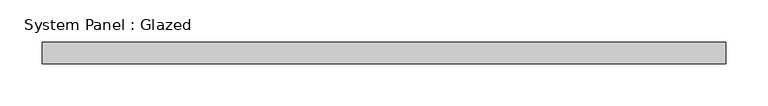
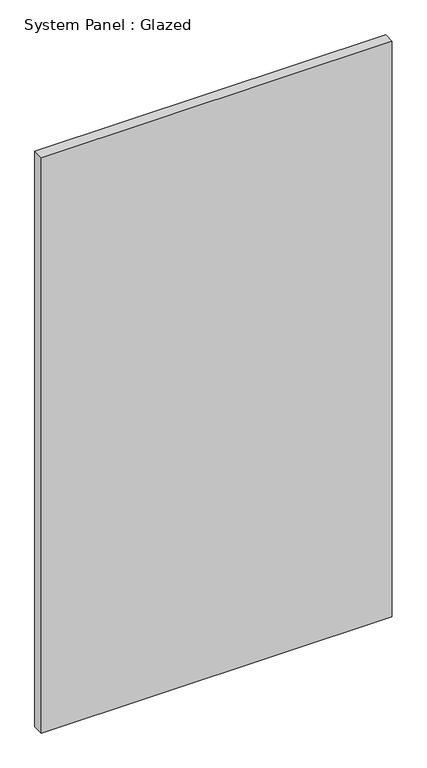
"""IFC4 building model written with IfcOpenShell, lengths in millimetres: plate geometry, System Panel : Glazed."""

from ifc_helpers import new_model, si_unit, origin, origin_with_axes, place, context, project, spatial, polyline, outline, extrude, source, transform, mapped, element, save


def system_panel_glazed_bdc0238d(model_context):
    return source(origin(), model_context, "Body", "SweptSolid", [
        extrude(outline(polyline([(405.6117773, 19.05), (-405.6117773, 19.05), (-405.6117773, 44.45), (405.6117773, 44.45), (405.6117773, 19.05)])), origin_with_axes(), (0.0, 0.0, 1.0), 1405.6819),
    ])


if __name__ == "__main__":
    model = new_model("IFC4")
    model_context = context("Model", 3, world=origin())
    ifc_project = project(units=[si_unit("LENGTHUNIT", "METRE", prefix="MILLI")], contexts=[model_context])
    site = spatial("IfcSite", under=ifc_project)
    building = spatial("IfcBuilding", under=site)
    placement = place(None, origin())
    system_panel_glazed_shape = system_panel_glazed_bdc0238d(model_context)
    element("IfcPlate", 1, ObjectType="System Panel : Glazed", at=placement, inside=building, context=model_context, shape_type="MappedRepresentation", body=[
        mapped(system_panel_glazed_shape, transform((0.0, 0.0, 0.0), x_axis=(1.0, 0.0, 0.0), y_axis=(0.0, 1.0, 0.0), z_axis=(0.0, 0.0, 1.0))),
    ])
    save(model, "model.ifc")

# Revit data of these elements
# Type "System Panel : Glazed"
#   Construction Type Id = "GSP4R"
#   Analytic Construction = "1/8 in Pilkington single glazing"
#   Visual Light Transmittance = 0.9
#   Solar Heat Gain Coefficient = 0.86
#   Heat Transfer Coefficient (U) = 1.18115 BTU/(h·ft²·°F)
#   Define Thermal Properties by = 1
# Element 1 (IfcPlate, "System Panel : Glazed")
#   Materials on its faces: "Glass"
# Materials
#   "Glass": class "Glass", colour RGB 0 128 192, transparency 0.75, Description = "Soda Lime Glass", Cost = 0
